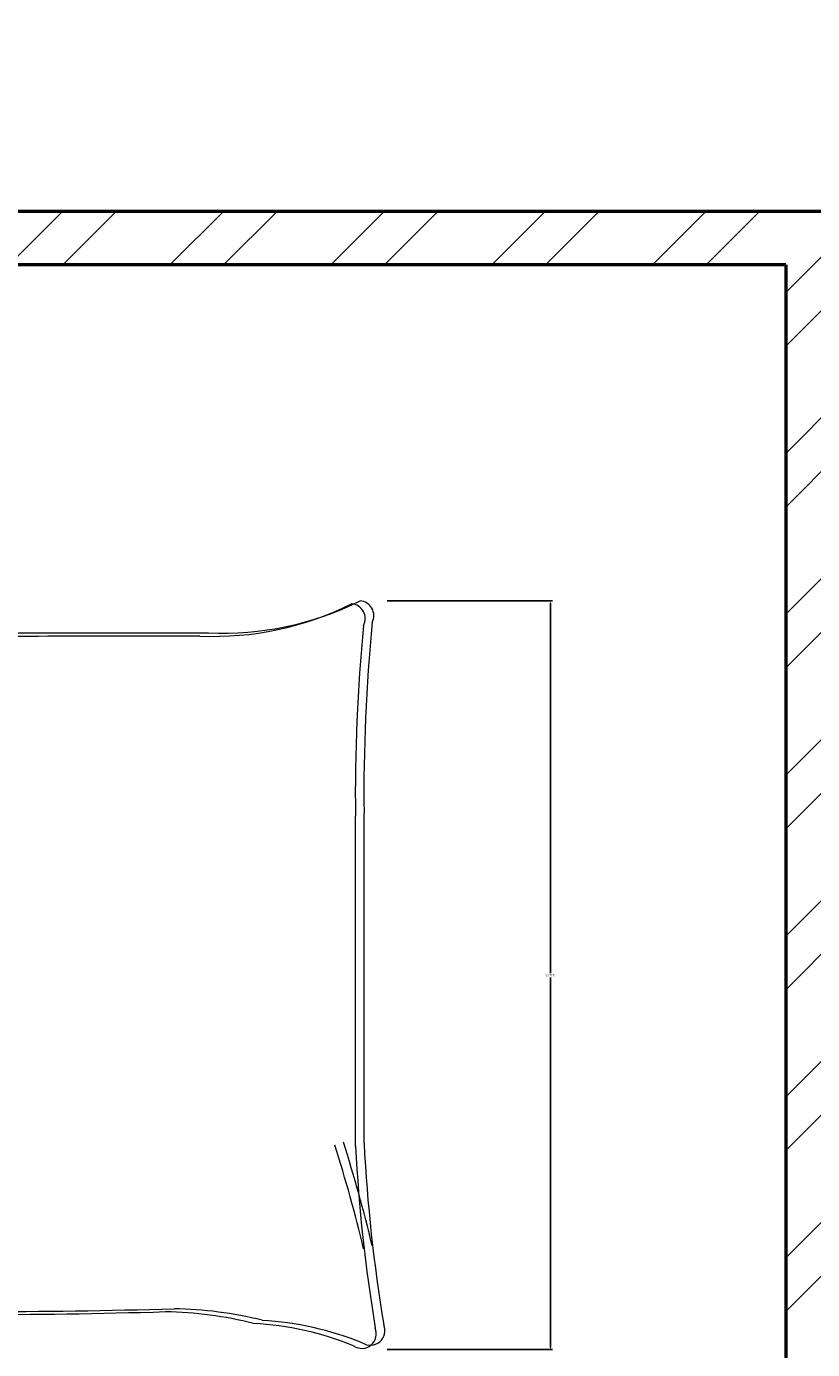
# Model space of a CAD drawing. Units: inches. Extents: x 1901 to 2863, y 888 to 2433.
# Tile 17 of 91: x 2091 to 2157, y 1621 to 1732. Entities that reach past the tile are written whole.
import ezdxf

# ---------------------------------------------------------------- set-up
doc = ezdxf.new("R2010")
doc.units = ezdxf.units.IN
for name, color, linetype, lineweight in [('A-ANNO-DIMS', 2, 'Continuous', 18), ('A-FURN', 8, 'Continuous', 18), ('A-WALL', 7, 'Continuous', 50), ('A-WALL-PATT', 8, 'Continuous', 13)]:
    doc.layers.add(name, color=color, linetype=linetype, lineweight=lineweight)
doc.styles.get("Standard").update_dxf_attribs({"font": 'arial.ttf'})
doc.dimstyles.get("Standard").update_dxf_attribs({"dimtxt": 0.18, "dimasz": 0.18, "dimexe": 0.18, "dimexo": 0.0625, "dimgap": 0.09, "dimtad": 0, "dimtih": 1, "dimtoh": 1, "dimdec": 4, "dimzin": 0, "dimdsep": 46, "dimtxsty": 'Standard', "dimcen": 0.09, "dimadec": 0, "dimazin": 0, "dimtfac": 1, "dimtdec": 4, "dimtofl": 0, "dimtmove": 0, "dimatfit": 3, "dimfxl": 1, "dimtolj": 1, "dimtzin": 0, "dimarcsym": 0})

# ---------------------------------------------------------------- blocks, each defined once
blk = doc.blocks.new('BED-DOUBLE')
for p, q in [((89, 16.88), (89, 44.51)), ((89, 16.88), (89, 44.51)), ((89.72, 17.13), (89.72, 44.77)), ((89.72, 17.13), (89.72, 44.77))]:
    blk.add_line(p, q)
for centre, radius, start, end in [((77.12, 85.47), 25.9, 267.4714, 296.4681), ((77.12, 85.47), 25.9, 267.4714, 296.4681), ((77.84, 85.73), 25.9, 267.4714, 296.4681), ((77.84, 85.73), 25.9, 267.4714, 296.4681), ((88.58, 61.05), 1.24, 332.6588, 86.02), ((88.58, 61.05), 1.24, 332.6588, 86.02), ((89.3, 61.31), 1.24, 332.6588, 86.02), ((89.3, 61.31), 1.24, 332.6588, 86.02), ((76.89, -5061.97), 5121.82, 90.00217, 90.28689), ((76.89, -5061.97), 5121.82, 90.00217, 90.28689), ((238.36, 46.17), 149.37, 174.4998, 180.6351), ((238.36, 46.17), 149.37, 174.4998, 180.6351), ((239.08, 46.42), 149.37, 174.4998, 180.6351), ((239.08, 46.42), 149.37, 174.4998, 180.6351), ((76.17, -5062.23), 5121.82, 90.00217, 90.28689), ((76.17, -5062.23), 5121.82, 90.00217, 90.28689), ((225.52, 24.02), 136.7, 182.9958, 189.4091), ((225.52, 24.02), 136.7, 182.9958, 189.4091), ((226.23, 24.28), 136.7, 182.9958, 189.4091), ((226.23, 24.28), 136.7, 182.9958, 189.4091), ((56.85, 544.3), 541.51, 268.2277, 271.7185), ((56.85, 544.3), 541.51, 268.2277, 271.7185), ((57.57, 544.55), 541.51, 268.2277, 271.7185), ((57.57, 544.55), 541.51, 268.2277, 271.7185), ((72.46, -30.24), 33.27, 76.0648, 88.9113), ((72.46, -30.24), 33.27, 76.0648, 88.9113), ((73.18, -29.98), 33.27, 76.0648, 88.9113), ((73.18, -29.98), 33.27, 76.0648, 88.9113), ((79.65, -24.1), 26.45, 67.9751, 86.652), ((79.65, -24.1), 26.45, 67.9751, 86.652), ((78.93, -24.35), 26.45, 67.9751, 86.652), ((78.93, -24.35), 26.45, 67.9751, 86.652), ((89.53, 1.18), 1.22, 236.1736, 23.4781), ((89.53, 1.18), 1.22, 236.1736, 23.4781), ((90.25, 1.44), 1.22, 236.1736, 23.4781), ((90.25, 1.44), 1.22, 236.1736, 23.4781)]:
    blk.add_arc(centre, radius, start, end)
blk = doc.blocks.new('*D18')
at = {"layer": 'A-ANNO-DIMS', "color": 0, "lineweight": -2, "transparency": 16777216}
for p, q in [((2120.95, 1683.99), (2134.8, 1683.99)), ((2134.62, 1683.81), (2134.62, 1652.83)), ((2134.62, 1621.49), (2134.62, 1652.47)), ((2120.95, 1621.31), (2134.8, 1621.31))]:
    blk.add_line(p, q, dxfattribs=at)
at = {"layer": 'A-ANNO-DIMS', "color": 0, "transparency": 16777216}
for points in [[(2134.59, 1683.81), (2134.65, 1683.81), (2134.62, 1683.99)], [(2134.59, 1621.49), (2134.65, 1621.49), (2134.62, 1621.31)]]:
    blk.add_solid(points, dxfattribs=at)
at = {"layer": 'Defpoints', "color": 0, "transparency": 16777216}
for p in [(2120.88, 1683.99), (2134.62, 1683.99), (2120.88, 1621.31)]:
    blk.add_point(p, dxfattribs=at)
at = {"layer": 'A-ANNO-DIMS', "color": 0, "transparency": 16777216, "insert": (2134.62, 1652.65), "char_height": 0.18, "attachment_point": 5}
blk.add_mtext('\\A1;63 TYP.', dxfattribs=at)

msp = doc.modelspace()

# ---------------------------------------------------------------- hatches: boundary and pattern name
at = {"layer": 'A-WALL-PATT'}
h = msp.add_hatch(dxfattribs=at)
h.set_pattern_fill('ANSI32', color=256)
h.paths.add_polyline_path([(2182.93, 1716.63), (2024.93, 1716.63), (2024.93, 1681.7), (2029.33, 1681.7), (2029.33, 1712.13), (2154.33, 1712.13), (2154.33, 1580.13), (2148.52, 1580.13), (2148.52, 1577.88), (2148.52, 1575.63), (2194.93, 1575.63), (2194.93, 1580.13), (2158.83, 1580.13), (2158.83, 1712.13), (2182.93, 1712.13)])
h.paths.add_polyline_path([(2301.07, 1716.63), (2242.93, 1716.63), (2242.93, 1712.13), (2283.83, 1712.13), (2283.83, 1685.54), (2288.33, 1685.54), (2288.33, 1712.13), (2301.07, 1712.13)])
h.paths.add_polyline_path([(2288.33, 1600.41), (2286.08, 1600.41), (2283.83, 1600.41), (2283.83, 1580.13), (2270.6, 1580.13), (2270.6, 1575.63), (2288.33, 1575.63)])
h.paths.add_polyline_path([(2295.93, 1953.63), (2271.45, 1953.63), (2271.45, 1949.13), (2291.43, 1949.13), (2291.43, 1941.24), (2295.93, 1941.24)])
h.paths.add_polyline_path([(2098.38, 1244.13), (2082.33, 1244.13), (2082.33, 1302.13), (2086.52, 1302.13), (2086.52, 1306.63), (2067.46, 1306.63), (2067.46, 1302.13), (2077.83, 1302.13), (2077.83, 1239.63), (2098.38, 1239.63), (2098.38, 1241.88)])
h.paths.add_polyline_path([(2217.31, 1306.63), (2158.83, 1306.63), (2158.83, 1451.63), (2162.72, 1451.63), (2162.72, 1453.88), (2162.72, 1456.13), (2154.33, 1456.13), (2154.33, 1443.13), (2151.91, 1443.13), (2151.91, 1438.63), (2154.33, 1438.63), (2154.33, 1306.63), (2109.31, 1306.63), (2109.31, 1304.38), (2109.31, 1302.13), (2154.33, 1302.13), (2154.33, 1244.13), (2122.38, 1244.13), (2122.38, 1239.63), (2154.33, 1239.63), (2154.33, 1223.63), (2163.33, 1223.63), (2181.01, 1223.63), (2181.01, 1225.88), (2181.01, 1228.13), (2163.33, 1228.13), (2163.33, 1258.22), (2158.83, 1258.22), (2158.83, 1302.13), (2217.31, 1302.13)])
h.paths.add_polyline_path([(2259.99, 1306.63), (2238.3, 1306.63), (2238.3, 1304.38), (2238.3, 1302.13), (2242.83, 1302.13), (2242.83, 1228.13), (2205.01, 1228.13), (2205.01, 1223.63), (2247.33, 1223.63), (2247.33, 1302.13), (2259.99, 1302.13), (2259.99, 1304.38)])
h.paths.add_polyline_path([(2343.43, 1361.7), (2338.93, 1361.7), (2338.93, 1306.63), (2322.38, 1306.63), (2322.38, 1302.13), (2343.43, 1302.13)])
h.paths.add_polyline_path([(2343.43, 1470.4), (2338.93, 1470.4), (2338.93, 1456.13), (2193.73, 1456.13), (2193.73, 1453.88), (2193.73, 1451.63), (2338.93, 1451.63), (2338.93, 1421.7), (2343.43, 1421.7)])
h.paths.add_polyline_path([(2343.43, 1545.51), (2338.93, 1545.51), (2338.93, 1530.4), (2343.43, 1530.4)])
h.paths.add_polyline_path([(2029.33, 1466.83), (2024.93, 1466.83), (2024.93, 1409.82), (2029.33, 1409.82)])
h.paths.add_polyline_path([(2122.84, 1440.88), (2122.84, 1443.13), (2121.83, 1443.13), (2121.83, 1498.18), (2119.58, 1498.18), (2117.33, 1498.18), (2117.33, 1443.13), (2029.33, 1443.13), (2029.33, 1438.63), (2122.84, 1438.63)])
h.paths.add_polyline_path([(2029.33, 1543.05), (2024.93, 1543.05), (2024.93, 1502.83), (2029.33, 1502.83)])
h.paths.add_polyline_path([(2029.33, 1621.7), (2024.93, 1621.7), (2024.93, 1567.05), (2027.13, 1567.05), (2029.33, 1567.05), (2029.33, 1575.63), (2109.33, 1575.63), (2109.33, 1554.71), (2113.83, 1554.71), (2113.83, 1575.63), (2115.8, 1575.63), (2115.8, 1577.88), (2115.8, 1580.13), (2029.33, 1580.13)])
h.paths.add_polyline_path([(2121.83, 1527.63), (2117.33, 1527.63), (2113.83, 1527.63), (2113.83, 1533.01), (2111.58, 1533.01), (2109.33, 1533.01), (2109.33, 1527.63), (2029.33, 1527.63), (2029.33, 1523.13), (2117.33, 1523.13), (2117.33, 1519.43), (2121.83, 1519.43)])
h.paths.add_polyline_path([(2029.33, 1349.82), (2024.93, 1349.82), (2024.93, 1302.13), (2036.28, 1302.13), (2036.28, 1306.63), (2029.33, 1306.63)])

# ---------------------------------------------------------------- linework, layer by layer
at = {"layer": 'A-FURN'}
for centre in [(2002.7, 1602.07), (2002.7, 1602.07), (2003.42, 1602.33), (2003.42, 1602.33)]:
    msp.add_arc(centre, 119.53, 13.3832, 17.7053, dxfattribs=at)
at = {"layer": 'A-WALL'}
for p, q in [((2024.93, 1716.63), (2301.07, 1716.63)), ((2154.33, 1712.13), (2029.33, 1712.13)), ((2154.33, 1712.13), (2154.33, 1580.13))]:
    msp.add_line(p, q, dxfattribs=at)

# ---------------------------------------------------------------- block references
at = {"layer": 'A-FURN'}
msp.add_blockref('BED-DOUBLE', (2029.3, 1621.45), dxfattribs=at)

# ---------------------------------------------------------------- dimensions: what is measured, and where the dimension line sits
at = {"layer": 'A-ANNO-DIMS'}
dim = msp.add_linear_dim(base=(2134.62, 1683.99), p1=(2120.88, 1621.31), p2=(2120.88, 1683.99), angle=90, text='<> TYP.', dimstyle='Standard', override={"dimdec": 0, "dimlfac": 1, "dimrnd": 0, "dimzin": 0, "dimdsep": 46, "dimlunit": 2}, dxfattribs=at)
dim.commit()
dim.dimension.update_dxf_attribs({"geometry": '*D18', "text_midpoint": (2134.62, 1652.65)})

doc.saveas('drawing.dxf')
